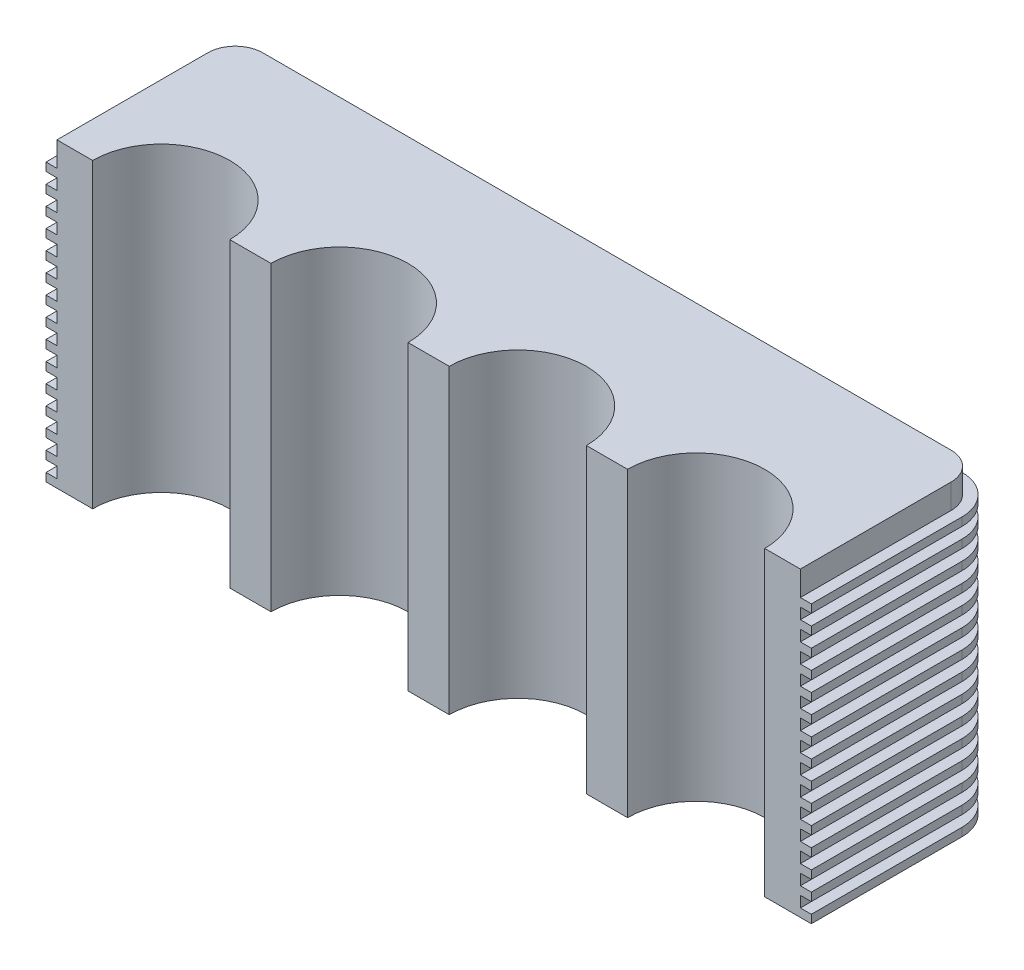
from build123d import *

# Parameters (mm, degrees)
UPPER_BLOCK_BODY_DEPTH             = 110
END_SERRATION_RIB_DEPTH            = 3
SERRATION_RIB_PATTERN_15X7MM_COUNT = 15
SERRATION_RIB_PATTERN_15X7MM_PITCH = 7


with BuildPart() as part:
    # Block Profile Sketch → Upper Block Body (new body)
    with BuildSketch(Plane(origin=(0, 0, 0), x_dir=(1, 0, 0), z_dir=(0, 1, 0))):
        with BuildLine():
            Line((0, 0), (13, 0))
            ThreePointArc((13, 0), (38, 25), (63, 0))
            Line((63, 0), (78, 0))
            ThreePointArc((78, 0), (103, 25), (128, 0))
            Line((128, 0), (143, 0))
            ThreePointArc((143, 0), (168, 25), (193, 0))
            Line((193, 0), (208, 0))
            ThreePointArc((208, 0), (233, 25), (258, 0))
            Line((258, 0), (271, 0))
            Line((271, 0), (271, 55))
            ThreePointArc((271, 55), (268.071067812, 62.071067812), (261, 65))
            Line((261, 65), (10, 65))
            ThreePointArc((10, 65), (2.928932188, 62.071067812), (0, 55))
            Line((0, 55), (0, 0))
        make_face()
    extrude(amount=UPPER_BLOCK_BODY_DEPTH)

    # End Serration Sketch → End Serration Rib (add)
    with BuildSketch(Plane(origin=(0, 0, 0), x_dir=(1, 0, 0), z_dir=(0, 1, 0))):
        with BuildLine():
            Line((275, 0), (275, 55))
            ThreePointArc((275, 55), (270.899494937, 64.899494937), (261, 69))
            Line((261, 69), (10, 69))
            ThreePointArc((10, 69), (0.100505063, 64.899494937), (-4, 55))
            Line((-4, 55), (-4, 0))
            Line((-4, 0), (0, 0))
            Line((0, 0), (0, 55))
            ThreePointArc((0, 55), (2.928932188, 62.071067812), (10, 65))
            Line((10, 65), (261, 65))
            ThreePointArc((261, 65), (268.071067812, 62.071067812), (271, 55))
            Line((271, 55), (271, 0))
            Line((271, 0), (275, 0))
        make_face()
    end_serration_rib = extrude(amount=END_SERRATION_RIB_DEPTH)

    # Serration Rib Pattern 15x7mm: End Serration Rib ×15
    with Locations(*[(0, i * SERRATION_RIB_PATTERN_15X7MM_PITCH, 0) for i in range(1, SERRATION_RIB_PATTERN_15X7MM_COUNT)]):
        add(end_serration_rib)


solid = part.part
